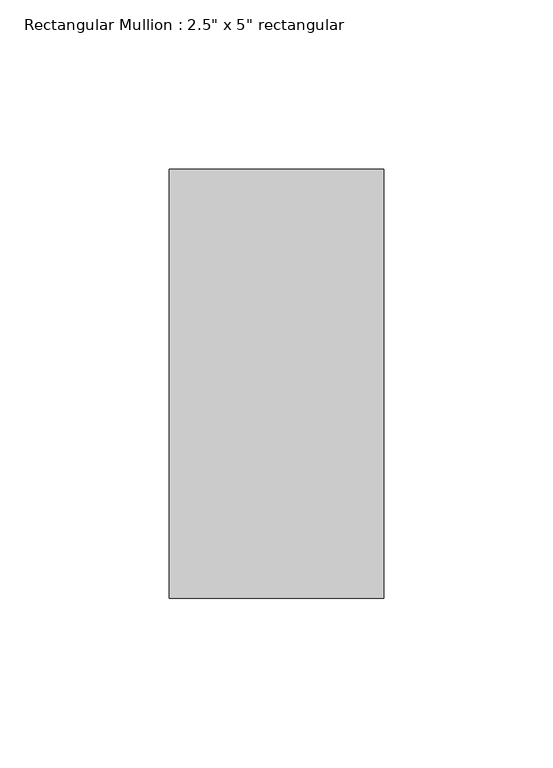
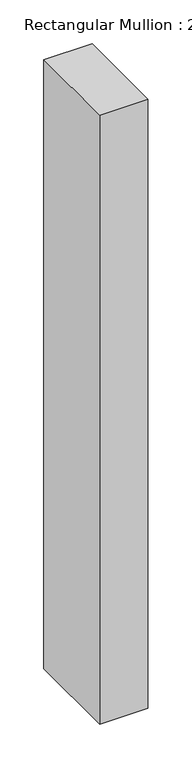
"""IFC4 building model written with IfcOpenShell, lengths in millimetres: member geometry."""

from ifc_helpers import new_model, si_unit, frame, origin, place, context, project, spatial, polyline, outline, extrude, source, transform, mapped, element, save


def member_63803c1e(model_context):
    return source(origin(), model_context, "Body", "SweptSolid", [
        extrude(outline(polyline([(31.75, 63.5), (31.75, -63.5), (-31.75, -63.5), (-31.75, 63.5), (31.75, 63.5)])), frame((0.0, 0.0, -848.0104839), z_axis=(0.0, 0.0, 1.0), x_axis=(1.0, 0.0, 0.0)), (0.0, 0.0, 1.0), 848.0104839),
    ])


if __name__ == "__main__":
    model = new_model("IFC4")
    model_context = context("Model", 3, world=origin())
    ifc_project = project(units=[si_unit("LENGTHUNIT", "METRE", prefix="MILLI")], contexts=[model_context])
    site = spatial("IfcSite", under=ifc_project)
    building = spatial("IfcBuilding", under=site)
    placement = place(None, origin())
    member_shape = member_63803c1e(model_context)
    element("IfcMember", 1, ObjectType="Rectangular Mullion : 2.5\" x 5\" rectangular", at=placement, inside=building, context=model_context, shape_type="MappedRepresentation", body=[
        mapped(member_shape, transform((0.0, 0.0, 0.0), x_axis=(1.0, 0.0, 0.0), y_axis=(0.0, 1.0, 0.0), z_axis=(0.0, 0.0, 1.0))),
    ])
    save(model, "model.ifc")

# Revit data of these elements
# Type "Rectangular Mullion : 2.5\" x 5\" rectangular"
#   built-in parameter 1007304 = 0.416667 (stored number, unit not read)
#   built-in parameter 1007301 = 0.104167 (stored number, unit not read)
#   built-in parameter 1007300 = 0.104167 (stored number, unit not read)
# Element 1 (IfcMember, "Rectangular Mullion : 2.5\" x 5\" rectangular")
#   Materials on its faces: "Aluminum"
# Materials
#   "Aluminum": class "Metal", colour RGB 247 247 247, transparency 0, Description = "Aluminum 6061", Cost = 0
